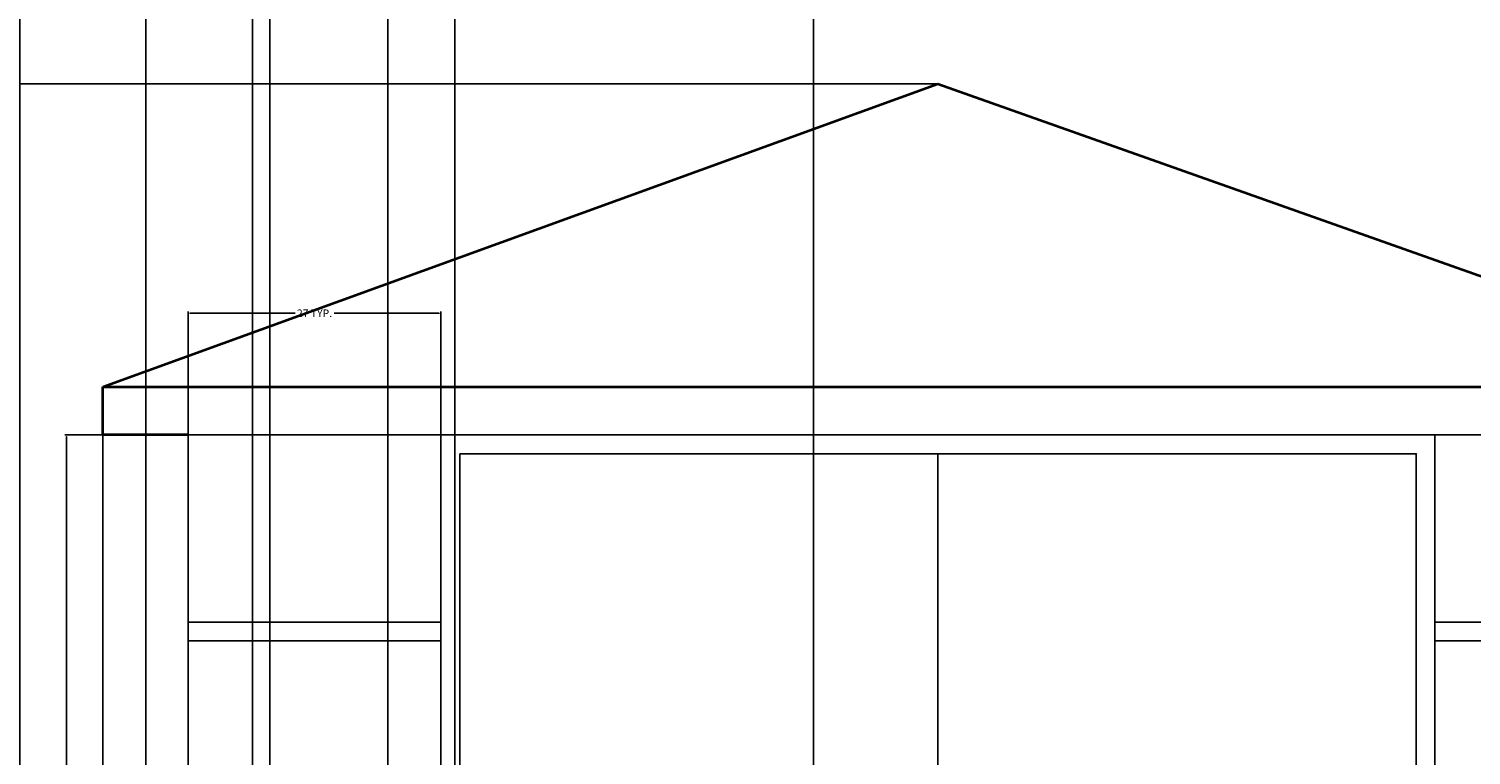
# Model space of a CAD drawing. Units: inches. Extents: x 69 to 650, y -16 to 573.
# Tile 8 of 26: x 345 to 499, y 140 to 218. Entities that reach past the tile are written whole.
import ezdxf

# ---------------------------------------------------------------- set-up
doc = ezdxf.new("R2010")
doc.units = ezdxf.units.IN
doc.header["$MEASUREMENT"] = 0
for name, color, linetype, lineweight in [('A-ANNO-DIMS', 2, 'Continuous', 18), ('A-COLS', 7, 'Continuous', 25), ('A-DOOR', 3, 'Continuous', 25), ('A-ROOF', 7, 'Continuous', 35)]:
    doc.layers.add(name, color=color, linetype=linetype, lineweight=lineweight)
doc.styles.get("Standard").update_dxf_attribs({"font": 'arial.ttf'})
doc.dimstyles.get("Standard").update_dxf_attribs({"dimtxt": 0.8125, "dimasz": 0.18, "dimexe": 0.18, "dimexo": 0.0625, "dimgap": 0.09, "dimtad": 0, "dimtih": 1, "dimtoh": 1, "dimdec": 4, "dimzin": 0, "dimdsep": 46, "dimlunit": 4, "dimtxsty": 'Standard', "dimcen": 0.09, "dimadec": 0, "dimazin": 0, "dimtfac": 1, "dimtdec": 4, "dimtofl": 0, "dimtmove": 0, "dimatfit": 3, "dimfxl": 1, "dimtolj": 1, "dimtzin": 0, "dimarcsym": 0})

# ---------------------------------------------------------------- blocks, each defined once
blk = doc.blocks.new('PIER-PORTAL-BANDED')
for p, q in [((0, 0), (0, 86.34)), ((0, 86.34), (26.94, 86.34)), ((0, 66.41), (26.94, 66.41)), ((0, 64.41), (26.94, 64.41)), ((0, 47.05), (26.94, 47.05)), ((0, 45.05), (26.94, 45.05)), ((0, 28.76), (26.94, 28.76)), ((0, 26.76), (26.94, 26.76)), ((0, 11.45), (26.94, 11.45)), ((0, 9.45), (26.94, 9.45))]:
    blk.add_line(p, q)
blk = doc.blocks.new('*D15')
at = {"layer": 'A-ANNO-DIMS', "color": 0, "lineweight": -2, "transparency": 16777216}
for p, q in [((361.96, 174.27), (348.89, 174.27)), ((349.07, 174.09), (349.07, 131.6)), ((349.07, 88.11), (349.07, 130.59)), ((361.96, 87.93), (348.89, 87.93))]:
    blk.add_line(p, q, dxfattribs=at)
at = {"layer": 'A-ANNO-DIMS', "color": 0, "transparency": 16777216}
for points in [[(349.04, 174.09), (349.1, 174.09), (349.07, 174.27)], [(349.04, 88.11), (349.1, 88.11), (349.07, 87.93)]]:
    blk.add_solid(points, dxfattribs=at)
at = {"layer": 'Defpoints', "color": 0, "transparency": 16777216}
for p in [(349.07, 174.27), (362.02, 174.27), (362.02, 87.93)]:
    blk.add_point(p, dxfattribs=at)
at = {"layer": 'A-ANNO-DIMS', "color": 0, "transparency": 16777216, "insert": (349.07, 131.1), "char_height": 0.8125, "attachment_point": 5}
blk.add_mtext('\\A1;PIER 86 TYP.', dxfattribs=at)
blk = doc.blocks.new('*D16')
at = {"layer": 'A-ANNO-DIMS', "color": 0, "lineweight": -2, "transparency": 16777216}
for p, q in [((362.02, 174.33), (362.02, 187.4)), ((362.2, 187.22), (373.42, 187.22)), ((388.78, 187.22), (377.57, 187.22)), ((388.96, 174.33), (388.96, 187.4))]:
    blk.add_line(p, q, dxfattribs=at)
at = {"layer": 'A-ANNO-DIMS', "color": 0, "transparency": 16777216}
for points in [[(362.2, 187.25), (362.2, 187.19), (362.02, 187.22)], [(388.78, 187.25), (388.78, 187.19), (388.96, 187.22)]]:
    blk.add_solid(points, dxfattribs=at)
at = {"layer": 'Defpoints', "color": 0, "transparency": 16777216}
for p in [(388.96, 187.22), (362.02, 174.27), (388.96, 174.27)]:
    blk.add_point(p, dxfattribs=at)
at = {"layer": 'A-ANNO-DIMS', "color": 0, "transparency": 16777216, "insert": (375.49, 187.22), "char_height": 0.8125, "attachment_point": 5}
blk.add_mtext('\\A1;27 TYP.', dxfattribs=at)
blk = doc.blocks.new('*D19')
at = {"layer": 'A-ANNO-DIMS', "color": 0, "lineweight": -2, "transparency": 16777216}
for p, q in [((99.56, 471.72), (99.56, 572.74)), ((99.74, 572.56), (358.57, 572.56)), ((619.38, 572.56), (360.54, 572.56)), ((619.56, 87.99), (619.56, 572.74))]:
    blk.add_line(p, q, dxfattribs=at)
at = {"layer": 'A-ANNO-DIMS', "color": 0, "transparency": 16777216}
for points in [[(99.74, 572.59), (99.74, 572.53), (99.56, 572.56)], [(619.38, 572.59), (619.38, 572.53), (619.56, 572.56)]]:
    blk.add_solid(points, dxfattribs=at)
at = {"layer": 'Defpoints', "color": 0, "transparency": 16777216}
for p in [(619.56, 572.56), (99.56, 471.66), (619.56, 87.93)]:
    blk.add_point(p, dxfattribs=at)
at = {"layer": 'A-ANNO-DIMS', "color": 0, "transparency": 16777216, "insert": (359.56, 572.56), "char_height": 0.812, "attachment_point": 5}
blk.add_mtext('\\A1;520', dxfattribs=at)
blk = doc.blocks.new('*D24')
at = {"layer": 'A-ANNO-DIMS', "color": 0, "lineweight": -2, "transparency": 16777216}
for p, q in [((441.88, 211.65), (70.98, 211.65)), ((71.16, 211.47), (71.16, 207.04)), ((71.16, 201.6), (71.16, 206.03)), ((173.51, 201.42), (70.98, 201.42))]:
    blk.add_line(p, q, dxfattribs=at)
at = {"layer": 'A-ANNO-DIMS', "color": 0, "transparency": 16777216}
for points in [[(71.13, 211.47), (71.19, 211.47), (71.16, 211.65)], [(71.13, 201.6), (71.19, 201.6), (71.16, 201.42)]]:
    blk.add_solid(points, dxfattribs=at)
at = {"layer": 'Defpoints', "color": 0, "transparency": 16777216}
for p in [(71.16, 211.65), (441.94, 211.65), (173.58, 201.42)]:
    blk.add_point(p, dxfattribs=at)
at = {"layer": 'A-ANNO-DIMS', "color": 0, "transparency": 16777216, "insert": (71.16, 206.54), "char_height": 0.812, "attachment_point": 5}
blk.add_mtext('\\A1;10.229', dxfattribs=at)
blk = doc.blocks.new('*D25')
at = {"layer": 'A-ANNO-DIMS', "color": 0, "lineweight": -2, "transparency": 16777216}
for p, q in [((99.49, 243.93), (70.98, 243.93)), ((71.16, 243.75), (71.16, 228.3)), ((71.16, 211.83), (71.16, 227.29)), ((441.88, 211.65), (70.98, 211.65))]:
    blk.add_line(p, q, dxfattribs=at)
at = {"layer": 'A-ANNO-DIMS', "color": 0, "transparency": 16777216}
for points in [[(71.13, 243.75), (71.19, 243.75), (71.16, 243.93)], [(71.13, 211.83), (71.19, 211.83), (71.16, 211.65)]]:
    blk.add_solid(points, dxfattribs=at)
at = {"layer": 'Defpoints', "color": 0, "transparency": 16777216}
for p in [(71.16, 243.93), (99.56, 243.93), (441.94, 211.65)]:
    blk.add_point(p, dxfattribs=at)
at = {"layer": 'A-ANNO-DIMS', "color": 0, "transparency": 16777216, "insert": (71.16, 227.79), "char_height": 0.812, "attachment_point": 5}
blk.add_mtext('\\A1;32.28', dxfattribs=at)
blk = doc.blocks.new('*D30')
at = {"layer": 'A-ANNO-DIMS', "color": 0, "lineweight": -2, "transparency": 16777216}
for p, q in [((352.94, 174.2), (352.94, 35.35)), ((313.14, 87.92), (313.14, 35.35)), ((313.32, 35.53), (331.9, 35.53)), ((352.76, 35.53), (334.19, 35.53))]:
    blk.add_line(p, q, dxfattribs=at)
at = {"layer": 'A-ANNO-DIMS', "color": 0, "transparency": 16777216}
for points in [[(313.32, 35.56), (313.32, 35.5), (313.14, 35.53)], [(352.76, 35.56), (352.76, 35.5), (352.94, 35.53)]]:
    blk.add_solid(points, dxfattribs=at)
at = {"layer": 'Defpoints', "color": 0, "transparency": 16777216}
for p in [(352.94, 174.27), (313.14, 87.99), (352.94, 35.53)]:
    blk.add_point(p, dxfattribs=at)
at = {"layer": 'A-ANNO-DIMS', "color": 0, "transparency": 16777216, "insert": (333.04, 35.53), "char_height": 0.812, "attachment_point": 5}
blk.add_mtext('\\A1;39.8', dxfattribs=at)
blk = doc.blocks.new('*D31')
at = {"layer": 'A-ANNO-DIMS', "color": 0, "lineweight": -2, "transparency": 16777216}
for p, q in [((352.94, 174.2), (352.94, 35.35)), ((362.02, 87.87), (362.02, 35.35)), ((353.12, 35.53), (356.1, 35.53)), ((361.84, 35.53), (358.86, 35.53))]:
    blk.add_line(p, q, dxfattribs=at)
at = {"layer": 'A-ANNO-DIMS', "color": 0, "transparency": 16777216}
for points in [[(353.12, 35.56), (353.12, 35.5), (352.94, 35.53)], [(361.84, 35.56), (361.84, 35.5), (362.02, 35.53)]]:
    blk.add_solid(points, dxfattribs=at)
at = {"layer": 'Defpoints', "color": 0, "transparency": 16777216}
for p in [(352.94, 174.27), (362.02, 87.93), (362.02, 35.53)]:
    blk.add_point(p, dxfattribs=at)
at = {"layer": 'A-ANNO-DIMS', "color": 0, "transparency": 16777216, "insert": (357.48, 35.53), "char_height": 0.812, "attachment_point": 5}
blk.add_mtext('\\A1;9.081', dxfattribs=at)
blk = doc.blocks.new('*D38')
at = {"layer": 'A-ANNO-DIMS', "color": 0, "lineweight": -2, "transparency": 16777216}
for p, q in [((307.8, 384.84), (307.8, 35.35)), ((390.43, 384.84), (390.43, 35.35)), ((307.98, 35.53), (347.65, 35.53)), ((390.25, 35.53), (350.57, 35.53))]:
    blk.add_line(p, q, dxfattribs=at)
at = {"layer": 'A-ANNO-DIMS', "color": 0, "transparency": 16777216}
for points in [[(307.98, 35.56), (307.98, 35.5), (307.8, 35.53)], [(390.25, 35.56), (390.25, 35.5), (390.43, 35.53)]]:
    blk.add_solid(points, dxfattribs=at)
at = {"layer": 'Defpoints', "color": 0, "transparency": 16777216}
for p in [(307.8, 384.9), (390.43, 384.9), (390.43, 35.53)]:
    blk.add_point(p, dxfattribs=at)
at = {"layer": 'A-ANNO-DIMS', "color": 0, "transparency": 16777216, "insert": (349.11, 35.53), "char_height": 0.812, "attachment_point": 5}
blk.add_mtext('\\A1;82.63', dxfattribs=at)
blk = doc.blocks.new('*D39')
at = {"layer": 'A-ANNO-DIMS', "color": 0, "lineweight": -2, "transparency": 16777216}
for p, q in [((390.43, 384.84), (390.43, 35.35)), ((428.66, 372.93), (428.66, 35.35)), ((390.61, 35.53), (407.77, 35.53)), ((428.48, 35.53), (411.32, 35.53))]:
    blk.add_line(p, q, dxfattribs=at)
at = {"layer": 'A-ANNO-DIMS', "color": 0, "transparency": 16777216}
for points in [[(390.61, 35.56), (390.61, 35.5), (390.43, 35.53)], [(428.48, 35.56), (428.48, 35.5), (428.66, 35.53)]]:
    blk.add_solid(points, dxfattribs=at)
at = {"layer": 'Defpoints', "color": 0, "transparency": 16777216}
for p in [(390.43, 384.9), (428.66, 372.99), (428.66, 35.53)]:
    blk.add_point(p, dxfattribs=at)
at = {"layer": 'A-ANNO-DIMS', "color": 0, "transparency": 16777216, "insert": (409.55, 35.53), "char_height": 0.812, "attachment_point": 5}
blk.add_mtext('\\A1;38.236', dxfattribs=at)
blk = doc.blocks.new('*D65')
at = {"layer": 'A-ANNO-DIMS', "color": 0, "lineweight": -2, "transparency": 16777216}
for p, q in [((344.08, 393.8), (344.08, 35.35)), ((368.88, 393.8), (368.88, 35.35)), ((344.26, 35.53), (355.33, 35.53)), ((368.7, 35.53), (357.63, 35.53))]:
    blk.add_line(p, q, dxfattribs=at)
at = {"layer": 'A-ANNO-DIMS', "color": 0, "transparency": 16777216}
for points in [[(344.26, 35.56), (344.26, 35.5), (344.08, 35.53)], [(368.7, 35.56), (368.7, 35.5), (368.88, 35.53)]]:
    blk.add_solid(points, dxfattribs=at)
at = {"layer": 'Defpoints', "color": 0, "transparency": 16777216}
for p in [(344.08, 393.86), (368.88, 393.86), (368.88, 35.53)]:
    blk.add_point(p, dxfattribs=at)
at = {"layer": 'A-ANNO-DIMS', "color": 0, "transparency": 16777216, "insert": (356.48, 35.53), "char_height": 0.812, "attachment_point": 5}
blk.add_mtext('\\A1;24.8', dxfattribs=at)
blk = doc.blocks.new('*D69')
at = {"layer": 'A-ANNO-DIMS', "color": 0, "lineweight": -2, "transparency": 16777216}
for p, q in [((343.89, 263.46), (343.89, 35.35)), ((357.51, 263.46), (357.51, 35.35)), ((344.07, 35.53), (349.28, 35.53)), ((357.33, 35.53), (352.12, 35.53))]:
    blk.add_line(p, q, dxfattribs=at)
at = {"layer": 'A-ANNO-DIMS', "color": 0, "transparency": 16777216}
for points in [[(344.07, 35.56), (344.07, 35.5), (343.89, 35.53)], [(357.33, 35.56), (357.33, 35.5), (357.51, 35.53)]]:
    blk.add_solid(points, dxfattribs=at)
at = {"layer": 'Defpoints', "color": 0, "transparency": 16777216}
for p in [(343.89, 263.53), (357.51, 263.53), (357.51, 35.53)]:
    blk.add_point(p, dxfattribs=at)
at = {"layer": 'A-ANNO-DIMS', "color": 0, "transparency": 16777216, "insert": (350.7, 35.53), "char_height": 0.812, "attachment_point": 5}
blk.add_mtext('\\A1;13.62', dxfattribs=at)
blk = doc.blocks.new('*D70')
at = {"layer": 'A-ANNO-DIMS', "color": 0, "lineweight": -2, "transparency": 16777216}
for p, q in [((357.51, 263.46), (357.51, 35.35)), ((370.73, 263.46), (370.73, 35.35)), ((357.69, 35.53), (362.46, 35.53)), ((370.55, 35.53), (365.78, 35.53))]:
    blk.add_line(p, q, dxfattribs=at)
at = {"layer": 'A-ANNO-DIMS', "color": 0, "transparency": 16777216}
for points in [[(357.69, 35.56), (357.69, 35.5), (357.51, 35.53)], [(370.55, 35.56), (370.55, 35.5), (370.73, 35.53)]]:
    blk.add_solid(points, dxfattribs=at)
at = {"layer": 'Defpoints', "color": 0, "transparency": 16777216}
for p in [(357.51, 263.53), (370.73, 263.53), (370.73, 35.53)]:
    blk.add_point(p, dxfattribs=at)
at = {"layer": 'A-ANNO-DIMS', "color": 0, "transparency": 16777216, "insert": (364.12, 35.53), "char_height": 0.812, "attachment_point": 5}
blk.add_mtext('\\A1;13.221', dxfattribs=at)
blk = doc.blocks.new('*D71')
at = {"layer": 'A-ANNO-DIMS', "color": 0, "lineweight": -2, "transparency": 16777216}
for p, q in [((370.73, 263.46), (370.73, 35.35)), ((383.3, 263.46), (383.3, 35.35)), ((370.91, 35.53), (375.59, 35.53)), ((383.12, 35.53), (378.44, 35.53))]:
    blk.add_line(p, q, dxfattribs=at)
at = {"layer": 'A-ANNO-DIMS', "color": 0, "transparency": 16777216}
for points in [[(370.91, 35.56), (370.91, 35.5), (370.73, 35.53)], [(383.12, 35.56), (383.12, 35.5), (383.3, 35.53)]]:
    blk.add_solid(points, dxfattribs=at)
at = {"layer": 'Defpoints', "color": 0, "transparency": 16777216}
for p in [(370.73, 263.53), (383.3, 263.53), (383.3, 35.53)]:
    blk.add_point(p, dxfattribs=at)
at = {"layer": 'A-ANNO-DIMS', "color": 0, "transparency": 16777216, "insert": (377.02, 35.53), "char_height": 0.812, "attachment_point": 5}
blk.add_mtext('\\A1;12.57', dxfattribs=at)

msp = doc.modelspace()

# ---------------------------------------------------------------- linework, layer by layer
at = {"layer": 'A-DOOR'}
msp.add_line((441.9398, 172.2666), (441.9398, 89.93), dxfattribs=at)
for points in [[(388.9646, 174.2666), (494.915, 174.2666), (494.915, 87.93), (388.9646, 87.93)], [(390.9646, 172.2666), (492.915, 172.2666), (492.915, 89.93), (390.9646, 89.93)]]:
    msp.add_lwpolyline(points, close=True, dxfattribs=at)
at = {"layer": 'A-ROOF'}
for p, q in [((352.9415, 179.3737), (441.9398, 211.6519)), ((441.9398, 211.6519), (533.1369, 179.3737)), ((352.9415, 174.2666), (352.9415, 179.3737)), ((352.9415, 179.3737), (533.1369, 179.3737)), ((362.0229, 174.2666), (352.9415, 174.2666))]:
    msp.add_line(p, q, dxfattribs=at)

# ---------------------------------------------------------------- block references
at = {"layer": 'A-COLS'}
msp.add_blockref('PIER-PORTAL-BANDED', (362.023, 87.93), dxfattribs=at)
at = {"layer": 'A-COLS', "extrusion": (0, 0, -1), "zscale": -1}
msp.add_blockref('PIER-PORTAL-BANDED', (-521.8566, 87.93), dxfattribs=at)

# ---------------------------------------------------------------- dimensions: what is measured, and where the dimension line sits
at = {"layer": 'A-ANNO-DIMS'}
for base, p1, p2, override, picture, middle in [((619.555, 572.5573), (99.556, 471.6595), (619.555, 87.93), {"dimdec": 0, "dimlfac": 1, "dimrnd": 0, "dimzin": 0, "dimdsep": 46, "dimlunit": 2}, '*D19', (359.5555, 572.5573)), ((368.881, 35.53), (344.0804, 393.8576), (368.881, 393.8576), {"dimdec": 1, "dimlfac": 1, "dimrnd": 0, "dimzin": 0, "dimdsep": 46, "dimlunit": 2}, '*D65', (356.4807, 35.53)), ((390.4291, 35.53), (307.7955, 384.8986), (390.4291, 384.8986), {"dimdec": 2, "dimlfac": 1, "dimrnd": 0, "dimzin": 0, "dimdsep": 46, "dimlunit": 2}, '*D38', (349.1123, 35.53)), ((428.6648, 35.53), (390.4291, 384.8986), (428.6648, 372.9907), {"dimdec": 3, "dimlfac": 1, "dimrnd": 0, "dimzin": 0, "dimdsep": 46, "dimlunit": 2}, '*D39', (409.547, 35.53)), ((357.5106, 35.53), (343.8902, 263.5253), (357.5106, 263.5253), {"dimdec": 2, "dimlfac": 1, "dimrnd": 0, "dimzin": 0, "dimdsep": 46, "dimlunit": 2}, '*D69', (350.7004, 35.53)), ((370.7319, 35.53), (357.5106, 263.5253), (370.7319, 263.5253), {"dimdec": 3, "dimlfac": 1, "dimrnd": 0, "dimzin": 0, "dimdsep": 46, "dimlunit": 2}, '*D70', (364.1213, 35.53)), ((383.3022, 35.53), (370.7319, 263.5253), (383.3022, 263.5253), {"dimdec": 2, "dimlfac": 1, "dimrnd": 0, "dimzin": 0, "dimdsep": 46, "dimlunit": 2}, '*D71', (377.0171, 35.53)), ((352.9415, 35.53), (313.1416, 87.985), (352.9415, 174.2666), {"dimdec": 1, "dimlfac": 1, "dimrnd": 0, "dimzin": 0, "dimdsep": 46, "dimlunit": 2}, '*D30', (333.0415, 35.53)), ((362.0229, 35.53), (352.9415, 174.2666), (362.0229, 87.93), {"dimdec": 3, "dimlfac": 1, "dimrnd": 0, "dimzin": 0, "dimdsep": 46, "dimlunit": 2}, '*D31', (357.4822, 35.53))]:
    dim = msp.add_linear_dim(base=base, p1=p1, p2=p2, dimstyle='Standard', override=override, dxfattribs=at)
    dim.commit()
    dim.dimension.update_dxf_attribs({"geometry": picture, "text_midpoint": middle})
for base, p1, p2, override, picture, middle in [((71.156, 243.93), (441.9398, 211.6519), (99.556, 243.93), {"dimdec": 2, "dimlfac": 1, "dimrnd": 0, "dimzin": 0, "dimdsep": 46, "dimlunit": 2}, '*D25', (71.156, 227.7909)), ((71.156, 211.6519), (173.5769, 201.4229), (441.9398, 211.6519), {"dimdec": 3, "dimlfac": 1, "dimrnd": 0, "dimzin": 0, "dimdsep": 46, "dimlunit": 2}, '*D24', (71.156, 206.5374))]:
    dim = msp.add_linear_dim(base=base, p1=p1, p2=p2, angle=90, dimstyle='Standard', override=override, dxfattribs=at)
    dim.commit()
    dim.dimension.update_dxf_attribs({"geometry": picture, "text_midpoint": middle})
dim = msp.add_linear_dim(base=(388.9646, 187.2171), p1=(362.0229, 174.2666), p2=(388.9646, 174.2666), text='<> TYP.', dimstyle='Standard', override={"dimdec": 0, "dimlfac": 1, "dimrnd": 0, "dimzin": 0, "dimdsep": 46, "dimlunit": 2}, dxfattribs=at)
dim.commit()
dim.dimension.update_dxf_attribs({"geometry": '*D16', "text_midpoint": (375.4938, 187.2171)})
dim = msp.add_linear_dim(base=(349.0724, 174.2666), p1=(362.0229, 87.93), p2=(362.0229, 174.2666), angle=90, text='PIER <> TYP.', dimstyle='Standard', override={"dimdec": 0, "dimlfac": 1, "dimrnd": 0, "dimzin": 0, "dimdsep": 46, "dimlunit": 2}, dxfattribs=at)
dim.commit()
dim.dimension.update_dxf_attribs({"geometry": '*D15', "text_midpoint": (349.0724, 131.0983)})

doc.saveas('drawing.dxf')
